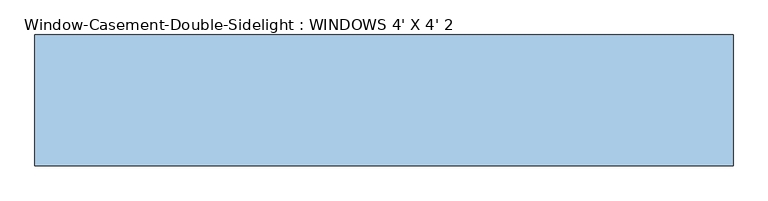
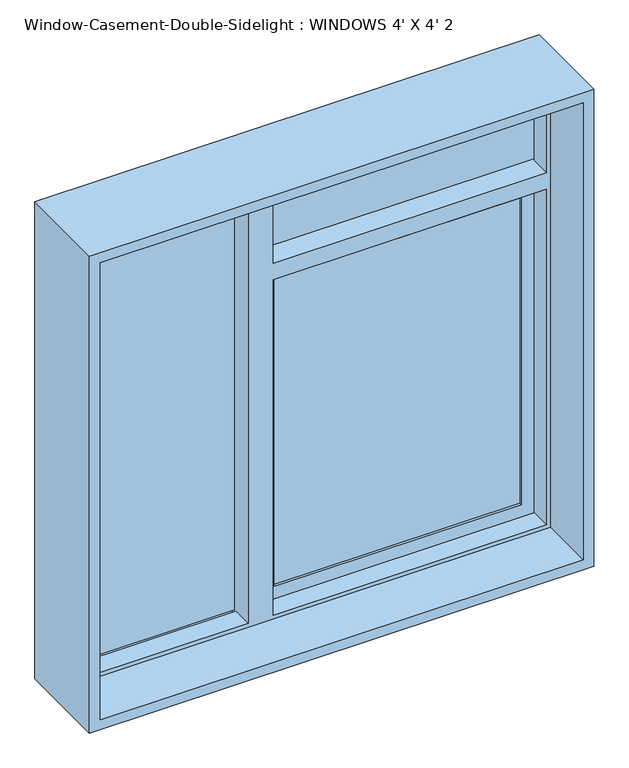
"""IFC4 building model written with IfcOpenShell, lengths in millimetres: window geometry, Window-Casement-Double-Sidelight : WINDOWS 4' X 4' 2."""

from ifc_helpers import new_model, si_unit, frame, origin, place, context, project, spatial, polyline, outline, extrude, faceted_brep, source, transform, mapped, element, save


def window_casement_double_sidelight_windows_4_x_4_2_a48be683(model_context):
    return source(origin(), model_context, "Body", "SolidModel", [
        extrude(outline(polyline([(542.3296875, 98.425), (-54.6496875, 98.425), (-54.6496875, 111.125), (542.3296875, 111.125), (542.3296875, 98.425)])), frame((0.0, 0.0, 981.6703125), z_axis=(0.0, 0.0, 1.0), x_axis=(1.0, 0.0, 0.0)), (0.0, 0.0, 1.0), 784.3242187),
        extrude(outline(polyline([(542.3296875, 85.725), (542.3296875, 79.375), (-54.6496875, 79.375), (-54.6496875, 85.725), (542.3296875, 85.725)])), frame((0.0, 0.0, 981.6703125), z_axis=(0.0, 0.0, 1.0), x_axis=(1.0, 0.0, 0.0)), (0.0, 0.0, 1.0), 784.3242187),
        extrude(outline(polyline([(-147.32, 98.425), (-147.32, 92.075), (-584.2, 92.075), (-584.2, 98.425), (-147.32, 98.425)])), frame((0.0, 0.0, 949.9203125), z_axis=(0.0, 0.0, 1.0), x_axis=(1.0, 0.0, 0.0)), (0.0, 0.0, 1.0), 1158.2796875),
        extrude(outline(polyline([(-147.32, 85.725), (-147.32, 79.375), (-584.2, 79.375), (-584.2, 85.725), (-147.32, 85.725)])), frame((0.0, 0.0, 949.9203125), z_axis=(0.0, 0.0, 1.0), x_axis=(1.0, 0.0, 0.0)), (0.0, 0.0, 1.0), 1158.2796875),
        extrude(outline(polyline([(584.2, 85.725), (584.2, 79.375), (-96.52, 79.375), (-96.52, 85.725), (584.2, 85.725)])), frame((0.0, 0.0, 1849.7351563), z_axis=(0.0, 0.0, 1.0), x_axis=(1.0, 0.0, 0.0)), (0.0, 0.0, 1.0), 258.4648438),
        extrude(outline(polyline([(584.2, 98.425), (584.2, 92.075), (-96.52, 92.075), (-96.52, 98.425), (584.2, 98.425)])), frame((0.0, 0.0, 1849.7351563), z_axis=(0.0, 0.0, 1.0), x_axis=(1.0, 0.0, 0.0)), (0.0, 0.0, 1.0), 258.4648438),
        faceted_brep([(-584.2, 73.025, 2108.2), (-584.2, 114.3, 2108.2), (584.2, 114.3, 2108.2), (584.2, 73.025, 2108.2), (-96.52, 73.025, 2108.2), (-96.52, 111.125, 2108.2), (-147.32, 111.125, 2108.2), (-147.32, 73.025, 2108.2), (-574.0796875, 22.225, 2098.0796875), (-574.0796875, 73.025, 2098.0796875), (-147.32, 73.025, 2098.0796875), (-147.32, 22.225, 2098.0796875), (574.0796875, 73.025, 2098.0796875), (574.0796875, 22.225, 2098.0796875), (-86.3996875, 22.225, 2098.0796875), (-86.3996875, 73.025, 2098.0796875), (-584.2, -114.3, 2108.2), (-584.2, 22.225, 2108.2), (584.2, 22.225, 2108.2), (584.2, -114.3, 2108.2), (-609.6, 114.3, 2133.6), (-609.6, -114.3, 2133.6), (609.6, -114.3, 2133.6), (609.6, 114.3, 2133.6), (584.2, 114.3, 939.8), (584.2, 73.025, 939.8), (584.2, 73.025, 1807.8648438), (584.2, 111.125, 1807.8648438), (584.2, 111.125, 1849.7351563), (584.2, 73.025, 1849.7351563), (574.0796875, 73.025, 1849.7351563), (574.0796875, 22.225, 1849.7351563), (574.0796875, 73.025, 949.9203125), (574.0796875, 22.225, 949.9203125), (574.0796875, 22.225, 1807.8648438), (574.0796875, 73.025, 1807.8648438), (584.2, 22.225, 939.8), (584.2, -114.3, 939.8), (609.6, -114.3, 914.4), (609.6, 114.3, 914.4), (-584.2, 114.3, 939.8), (-584.2, 73.025, 939.8), (-147.32, 73.025, 939.8), (-147.32, 111.125, 939.8), (-96.52, 111.125, 939.8), (-96.52, 73.025, 939.8), (-86.3996875, 73.025, 949.9203125), (-86.3996875, 22.225, 949.9203125), (-574.0796875, 73.025, 949.9203125), (-574.0796875, 22.225, 949.9203125), (-147.32, 22.225, 949.9203125), (-147.32, 73.025, 949.9203125), (-584.2, 22.225, 939.8), (-584.2, -114.3, 939.8), (-609.6, -114.3, 914.4), (-609.6, 114.3, 914.4), (-86.3996875, 73.025, 1849.7351563), (-96.52, 73.025, 1849.7351563), (-96.52, 73.025, 1807.8648438), (-86.3996875, 73.025, 1807.8648438), (-86.3996875, 22.225, 1849.7351563), (-86.3996875, 22.225, 1807.8648438), (-96.52, 111.125, 1849.7351563), (-96.52, 111.125, 1807.8648438)], [[[0, 1, 2, 3, 4, 5, 6, 7]], [[8, 9, 10, 11]], [[12, 13, 14, 15]], [[16, 17, 18, 19]], [[20, 21, 22, 23]], [[3, 2, 24, 25, 26, 27, 28, 29]], [[13, 12, 30, 31]], [[32, 33, 34, 35]], [[19, 18, 36, 37]], [[23, 22, 38, 39]], [[25, 24, 40, 41, 42, 43, 44, 45]], [[33, 32, 46, 47]], [[48, 49, 50, 51]], [[37, 36, 52, 53]], [[39, 38, 54, 55]], [[1, 0, 41, 40]], [[12, 15, 56, 57, 4, 3, 29, 30]], [[46, 32, 35, 26, 25, 45, 58, 59]], [[41, 0, 7, 10, 9, 48, 51, 42]], [[9, 8, 49, 48]], [[17, 52, 36, 18], [13, 31, 60, 14], [33, 47, 61, 34], [49, 8, 11, 50]], [[17, 16, 53, 52]], [[22, 21, 54, 38], [16, 19, 37, 53]], [[21, 20, 55, 54]], [[20, 23, 39, 55], [2, 1, 40, 24]], [[43, 6, 5, 62, 28, 27, 63, 44]], [[6, 43, 42, 51, 50, 11, 10, 7]], [[15, 14, 60, 56]], [[47, 46, 59, 61]], [[5, 4, 57, 62]], [[45, 44, 63, 58]], [[63, 27, 26, 35, 34, 61, 59, 58]], [[28, 62, 57, 56, 60, 31, 30, 29]]]),
        extrude(outline(polyline([(1807.8648438, 584.2), (1807.8648438, -96.52), (939.8, -96.52), (939.8, 584.2), (1807.8648438, 584.2)]), holes=[polyline([(981.6703125, 542.3296875), (981.6703125, -54.6496875), (1765.9945313, -54.6496875), (1765.9945313, 542.3296875), (981.6703125, 542.3296875)])]), frame((0.0, 73.025, 0.0), z_axis=(0.0, 1.0, 0.0), x_axis=(0.0, 0.0, 1.0)), (0.0, 0.0, 1.0), 31.75),
    ])


if __name__ == "__main__":
    model = new_model("IFC4")
    model_context = context("Model", 3, world=origin())
    ifc_project = project(units=[si_unit("LENGTHUNIT", "METRE", prefix="MILLI")], contexts=[model_context])
    site = spatial("IfcSite", under=ifc_project)
    building = spatial("IfcBuilding", under=site)
    placement = place(None, origin())
    window_casement_double_sidelight_windows_4_x_4_2_shape = window_casement_double_sidelight_windows_4_x_4_2_a48be683(model_context)
    element("IfcWindow", 1, ObjectType="Window-Casement-Double-Sidelight : WINDOWS 4' X 4' 2", at=placement, inside=building, context=model_context, shape_type="MappedRepresentation", body=[
        mapped(window_casement_double_sidelight_windows_4_x_4_2_shape, transform((0.0, 0.0, 0.0), x_axis=(1.0, 0.0, 0.0), y_axis=(0.0, 1.0, 0.0), z_axis=(0.0, 0.0, 1.0))),
    ])
    save(model, "model.ifc")

# Revit data of these elements
# Type "Window-Casement-Double-Sidelight : WINDOWS 4' X 4' 2"
#   Type Mark = "25"
#   Fire Rating = "0.5h"
#   Assembly Code = "B2020100"
#   Analytic Construction = "Double glazing - domestic"
#   Window Inset [instance default] = 0' - 0 5/8"
#   Wall Thickness [instance default] = 0' - 6"
#   Visual Light Transmittance = 0.81
#   Transom Height Ratio = 0.25
#   Transom Height = 1' - 0"
#   Thermal Resistance (R) = 1.8146 (h·ft²·°F)/BTU
#   Solar Heat Gain Coefficient = 0.76
#   Side Width = 1' - 7.2"
#   Rough Width = 4' - 0 1/2"
#   Rough Height = 4' - 0 1/2"
#   Opening Window Width = 2' - 4.8"
#   Opening Window Height = 3' - 0"
#   Heat Transfer Coefficient (U) = 0.5511 BTU/(h·ft²·°F)
#   Height = 4' - 0"
#   Frame Gap 3 [instance default] = 0' - 1 83/128"
#   Frame Gap 2 [instance default] = 0' - 0 5/8"
#   Frame Gap 1 = 0' - 1 51/128"
#   Default Sill Height = 3' - 0"
#   Width = 4' - 0"
#   Frame Material = BLACK MATERIAL
#   Glass Panel Material = Glass
#   Wall Closure = (empty or 0)
# Element 1 (IfcWindow, "Window-Casement-Double-Sidelight : WINDOWS 4' X 4' 2")
#   Wall Thickness = 0' - 9"
#   Materials on its faces: "BLACK MATERIAL", "Glass"
# Materials
#   "BLACK MATERIAL": class "Generic", colour RGB 120 120 120, transparency 0, Cost = 0
#   "Glass": class "Glass", colour RGB 0 128 192, transparency 0.75, Description = "Soda Lime Glass", Cost = 0
